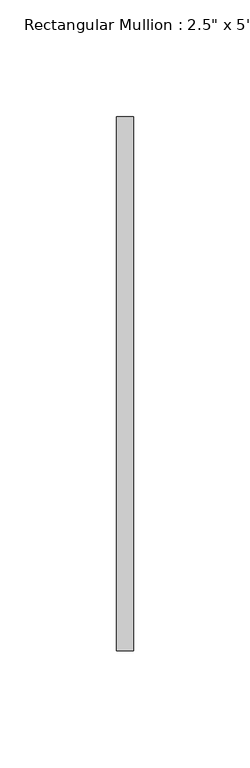
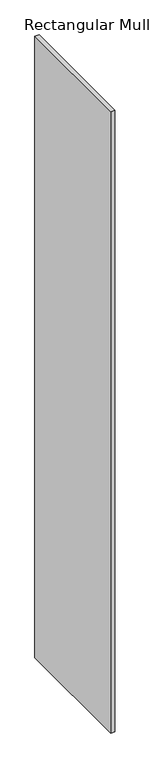
"""IFC4 building model written with IfcOpenShell, lengths in millimetres: member geometry."""

from ifc_helpers import new_model, si_unit, frame, origin, place, context, project, spatial, polyline, outline, extrude, source, transform, mapped, element, save


def member_fa9cb678(model_context):
    return source(origin(), model_context, "Body", "SweptSolid", [
        extrude(outline(polyline([(3.6195, 114.3), (3.6195, -114.3), (-3.6195, -114.3), (-3.6195, 114.3), (3.6195, 114.3)])), frame((0.0, 0.0, -1144.8415), z_axis=(0.0, 0.0, 1.0), x_axis=(1.0, 0.0, 0.0)), (0.0, 0.0, 1.0), 1144.8415),
    ])


if __name__ == "__main__":
    model = new_model("IFC4")
    model_context = context("Model", 3, world=origin())
    ifc_project = project(units=[si_unit("LENGTHUNIT", "METRE", prefix="MILLI")], contexts=[model_context])
    site = spatial("IfcSite", under=ifc_project)
    building = spatial("IfcBuilding", under=site)
    placement = place(None, origin())
    member_shape = member_fa9cb678(model_context)
    element("IfcMember", 1, ObjectType="Rectangular Mullion : 2.5\" x 5\" rectangular", at=placement, inside=building, context=model_context, shape_type="MappedRepresentation", body=[
        mapped(member_shape, transform((0.0, 0.0, 0.0), x_axis=(1.0, 0.0, 0.0), y_axis=(0.0, 1.0, 0.0), z_axis=(0.0, 0.0, 1.0))),
    ])
    save(model, "model.ifc")

# Revit data of these elements
# Type "Rectangular Mullion : 2.5\" x 5\" rectangular"
#   built-in parameter 1007304 = 0.75 (stored number, unit not read)
#   built-in parameter 1007301 = 0.011875 (stored number, unit not read)
#   built-in parameter 1007300 = 0.011875 (stored number, unit not read)
# Element 1 (IfcMember, "Rectangular Mullion : 2.5\" x 5\" rectangular")
#   Materials on its faces: "WINDOW GLASS MATERIAL"
# Materials
#   "WINDOW GLASS MATERIAL": class "Generic", colour RGB 120 120 120, transparency 0, Cost = 0
